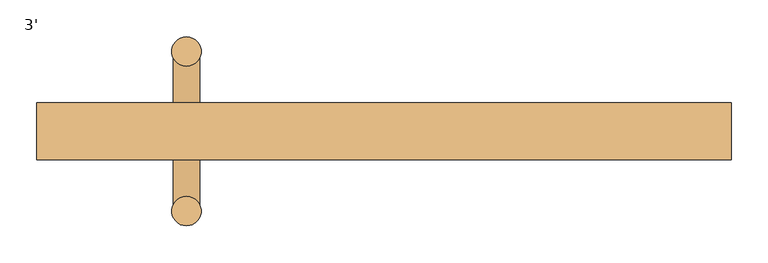
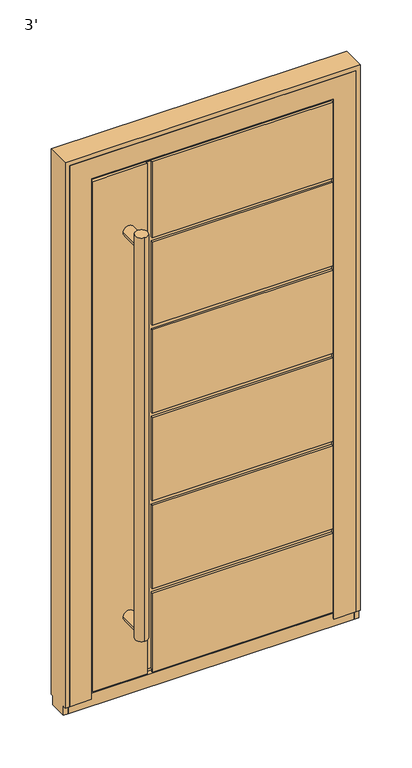
"""IFC4 building model written with IfcOpenShell, lengths in millimetres: door geometry, 3'."""

from ifc_helpers import new_model, si_unit, point, frame, frame_2d, origin, place, context, project, spatial, circle_curve, trimmed, segment, composite_curve, outline, extrude, faceted_brep, source, transform, mapped, element, save


def door_3_ad1505b7(model_context):
    return source(origin(), model_context, "Body", "SolidModel", [
        extrude(outline(composite_curve([segment(trimmed(circle_curve(frame_2d((-268.65, -90.8003001)), 20.0), [point((-268.65, -70.8003001))], [point((-268.65, -110.8003001))], False, "CARTESIAN"), True, "CONTINUOUS"), segment(trimmed(circle_curve(frame_2d((-268.65, -90.8003001)), 20.0), [point((-268.65, -110.8003001))], [point((-268.65, -70.8003001))], False, "CARTESIAN"), True, "CONTINUOUS")], self_intersect=False)), frame((0.0, 0.0, 210.0000003), z_axis=(0.0, 0.0, 1.0), x_axis=(1.0, 0.0, 0.0)), (0.0, 0.0, 1.0), 1363.8),
        extrude(outline(composite_curve([segment(trimmed(circle_curve(frame_2d((-268.65, 126.2003001)), 20.0), [point((-268.65, 146.2003001))], [point((-268.65, 106.2003001))], False, "CARTESIAN"), True, "CONTINUOUS"), segment(trimmed(circle_curve(frame_2d((-268.65, 126.2003001)), 20.0), [point((-268.65, 106.2003001))], [point((-268.65, 146.2003001))], False, "CARTESIAN"), True, "CONTINUOUS")], self_intersect=False)), frame((0.0, 0.0, 210.0000003), z_axis=(0.0, 0.0, 1.0), x_axis=(1.0, 0.0, 0.0)), (0.0, 0.0, 1.0), 1363.8),
        extrude(outline(composite_curve([segment(trimmed(circle_curve(frame_2d((241.9000003, -268.65)), 18.0), [point((241.9000003, -286.65))], [point((241.9000003, -250.65))], False, "CARTESIAN"), True, "CONTINUOUS"), segment(trimmed(circle_curve(frame_2d((241.9000003, -268.65)), 18.0), [point((241.9000003, -250.65))], [point((241.9000003, -286.65))], False, "CARTESIAN"), True, "CONTINUOUS")], self_intersect=False)), frame((0.0, -90.8, 0.0), z_axis=(0.0, 1.0, 0.0), x_axis=(0.0, 0.0, 1.0)), (0.0, 0.0, 1.0), 217.0),
        extrude(outline(composite_curve([segment(trimmed(circle_curve(frame_2d((1541.9000003, -268.65)), 18.0), [point((1541.9000003, -286.65))], [point((1541.9000003, -250.65))], False, "CARTESIAN"), True, "CONTINUOUS"), segment(trimmed(circle_curve(frame_2d((1541.9000003, -268.65)), 18.0), [point((1541.9000003, -250.65))], [point((1541.9000003, -286.65))], False, "CARTESIAN"), True, "CONTINUOUS")], self_intersect=False)), frame((0.0, -90.8, 0.0), z_axis=(0.0, 1.0, 0.0), x_axis=(0.0, 0.0, 1.0)), (0.0, 0.0, 1.0), 217.0),
        faceted_brep([(-193.65, -13.8, 306.466667), (-193.65, -13.8, 587.9333337), (383.65, -13.8, 587.9333337), (383.65, -13.8, 602.9333337), (-193.65, -13.8, 602.9333337), (-193.65, -13.8, 884.4000004), (383.65, -13.8, 884.4000004), (383.65, -13.8, 899.4000004), (-193.65, -13.8, 899.4000004), (-193.65, -13.8, 1180.866667), (383.65, -13.8, 1180.866667), (383.65, -13.8, 1195.866667), (-193.65, -13.8, 1195.866667), (-193.65, -13.8, 1477.3333337), (383.65, -13.8, 1477.3333337), (383.65, -13.8, 1492.3333337), (-193.65, -13.8, 1492.3333337), (-193.65, -13.8, 1748.8000003), (-208.65, -13.8, 1748.8000003), (-208.65, -13.8, 35.0), (-193.65, -13.8, 35.0), (-193.65, -13.8, 291.466667), (383.65, -13.8, 291.466667), (383.65, -13.8, 306.466667), (-193.65, -20.8, 306.466667), (-193.65, -20.8, 587.9333337), (383.65, -20.8, 587.9333337), (383.65, -11.7997698, 1748.8000003), (383.65, -20.8, 1748.8000003), (383.65, -20.8, 1492.3333337), (383.65, -20.8, 1477.3333337), (383.65, -20.8, 1195.866667), (383.65, -20.8, 1180.866667), (383.65, -20.8, 899.4000004), (383.65, -20.8, 884.4000004), (383.65, -20.8, 602.9333337), (383.65, -20.8, 306.466667), (383.65, -20.8, 291.466667), (383.65, -20.8, 24.0), (383.65, -18.8020472, 24.0), (383.65, -18.8020472, 35.0), (383.65, -11.7997698, 35.0), (-193.65, -20.8, 602.9333337), (-193.65, -20.8, 884.4000004), (-193.65, -20.8, 899.4000004), (-193.65, -20.8, 1180.866667), (-208.65, -20.8, 1748.8000003), (-208.65, -20.8, 24.0), (-208.65, -18.8020472, 24.0), (-208.65, -18.8020472, 35.0), (-193.65, -18.8020472, 35.0), (-383.65, -18.8020472, 35.0), (-383.65, -11.7997698, 35.0), (-193.65, -20.8, 291.466667), (-193.65, -18.8020472, 24.0), (-193.65, -20.8, 24.0), (-383.65, -18.8020472, 24.0), (-383.65, -20.8, 24.0), (-383.65, -20.8, 1748.8000003), (-193.65, -20.8, 1477.3333337), (-193.65, -20.8, 1195.866667), (-193.65, -20.8, 1748.8000003), (-193.65, -20.8, 1492.3333337), (408.65, 56.2, 10.0000003), (408.65, 53.2, 10.0000003), (-193.65, 53.2, 10.0000003), (-193.65, 56.2, 10.0000003), (-408.65, 53.2, 10.0000003), (-408.65, 56.2, 10.0000003), (-208.65, 56.2, 10.0000003), (-208.65, 53.2, 10.0000003), (408.65, 56.2, 291.466667), (408.65, 53.2, 291.466667), (408.65, 56.2, 306.466667), (408.65, 56.2, 587.9333337), (408.65, 53.2, 587.9333337), (408.65, 53.2, 306.466667), (408.65, 56.2, 899.4000004), (408.65, 56.2, 1180.866667), (408.65, 53.2, 1180.866667), (408.65, 53.2, 899.4000004), (408.65, 56.2, 602.9333337), (408.65, 56.2, 884.4000004), (408.65, 53.2, 884.4000004), (408.65, 53.2, 602.9333337), (408.65, 56.2, 1195.866667), (408.65, 56.2, 1477.3333337), (408.65, 53.2, 1477.3333337), (408.65, 53.2, 1195.866667), (408.65, 56.2, 1773.8000003), (408.65, 53.2, 1773.8000003), (408.65, 53.2, 1492.3333337), (408.65, 56.2, 1492.3333337), (393.15, 53.2, 291.466667), (393.15, 53.2, 25.5), (-193.65, 53.2, 25.5), (393.15, 53.2, 587.9333337), (393.15, 53.2, 306.466667), (393.15, 53.2, 1180.866667), (393.15, 53.2, 899.4000004), (393.15, 53.2, 884.4000004), (393.15, 53.2, 602.9333337), (393.15, 53.2, 1477.3333337), (393.15, 53.2, 1195.866667), (-193.65, 53.2, 1773.8000003), (-193.65, 53.2, 1758.3000003), (393.15, 53.2, 1758.3000003), (393.15, 53.2, 1492.3333337), (-393.15, 53.2, 25.5), (-393.15, 53.2, 1758.3000003), (-208.65, 53.2, 1758.3000003), (-208.65, 53.2, 1773.8000003), (-408.65, 53.2, 1773.8000003), (-208.65, 53.2, 25.5), (-193.65, 49.2, 291.466667), (-193.65, 56.2, 291.466667), (-193.65, 49.2, 25.5), (-193.65, 56.2, 306.466667), (-193.65, 56.2, 587.9333337), (-193.65, 56.2, 899.4000004), (-193.65, 56.2, 1180.866667), (-193.65, 56.2, 602.9333337), (-193.65, 56.2, 884.4000004), (-193.65, 56.2, 1195.866667), (-193.65, 56.2, 1477.3333337), (-193.65, 56.2, 1492.3333337), (-193.65, 56.2, 1773.8000003), (-408.65, 56.2, 1773.8000003), (-208.65, 56.2, 1773.8000003), (-208.65, 49.2, 1758.3000003), (-208.65, 49.2, 25.5), (-383.65, -11.7997698, 1748.8000003), (393.15, -11.7997698, 1758.3000003), (-393.15, -11.7997698, 1758.3000003), (-393.15, -11.7997698, 25.5), (393.15, -11.7997698, 25.5), (393.15, 49.2, 291.466667), (393.15, 49.2, 306.466667), (393.15, 49.2, 587.9333337), (393.15, 49.2, 602.9333337), (393.15, 49.2, 884.4000004), (393.15, 49.2, 899.4000004), (393.15, 49.2, 1180.866667), (393.15, 49.2, 1195.866667), (393.15, 49.2, 1477.3333337), (393.15, 49.2, 1492.3333337), (-193.65, 49.2, 1477.3333337), (-193.65, 49.2, 1195.866667), (-193.65, 49.2, 1180.866667), (-193.65, 49.2, 899.4000004), (-193.65, 49.2, 884.4000004), (-193.65, 49.2, 602.9333337), (-193.65, 49.2, 587.9333337), (-193.65, 49.2, 306.466667), (-193.65, 49.2, 1758.3000003), (-193.65, 49.2, 1492.3333337)], [[[0, 1, 2, 3, 4, 5, 6, 7, 8, 9, 10, 11, 12, 13, 14, 15, 16, 17, 18, 19, 20, 21, 22, 23]], [[1, 0, 24, 25]], [[1, 25, 26, 2]], [[27, 28, 29, 15, 14, 30, 31, 11, 10, 32, 33, 7, 6, 34, 35, 3, 2, 26, 36, 23, 22, 37, 38, 39, 40, 41]], [[42, 4, 3, 35]], [[5, 4, 42, 43]], [[5, 43, 34, 6]], [[44, 8, 7, 33]], [[9, 8, 44, 45]], [[19, 18, 46, 47, 48, 49]], [[41, 40, 50, 20, 19, 49, 51, 52]], [[53, 21, 20, 50, 54, 55]], [[21, 53, 37, 22]], [[24, 0, 23, 36]], [[40, 39, 54, 50]], [[56, 51, 49, 48]], [[39, 38, 55, 54]], [[57, 56, 48, 47]], [[33, 32, 45, 44]], [[35, 34, 43, 42]], [[36, 26, 25, 24]], [[55, 38, 37, 53]], [[58, 57, 47, 46]], [[31, 30, 59, 60]], [[28, 61, 62, 29]], [[63, 64, 65, 66]], [[67, 68, 69, 70]], [[64, 63, 71, 72]], [[73, 74, 75, 76]], [[77, 78, 79, 80]], [[81, 82, 83, 84]], [[85, 86, 87, 88]], [[89, 90, 91, 92]], [[65, 64, 72, 93, 94, 95]], [[76, 75, 96, 97]], [[80, 79, 98, 99]], [[84, 83, 100, 101]], [[88, 87, 102, 103]], [[90, 104, 105, 106, 107, 91]], [[108, 109, 110, 111, 112, 67, 70, 113]], [[114, 115, 66, 65, 95, 116]], [[63, 66, 115, 71]], [[74, 73, 117, 118]], [[78, 77, 119, 120]], [[82, 81, 121, 122]], [[86, 85, 123, 124]], [[89, 92, 125, 126]], [[68, 127, 128, 69]], [[68, 67, 112, 127]], [[129, 130, 113, 70, 69, 128, 111, 110]], [[58, 131, 52, 51, 56, 57]], [[132, 133, 134, 135], [131, 27, 41, 52]], [[106, 132, 135, 94, 93, 136, 137, 97, 96, 138, 139, 101, 100, 140, 141, 99, 98, 142, 143, 103, 102, 144, 145, 107]], [[94, 135, 134, 108, 113, 130, 116, 95]], [[133, 109, 108, 134]], [[146, 147, 143, 142, 148, 149, 141, 140, 150, 151, 139, 138, 152, 153, 137, 136, 114, 116, 130, 129, 154, 155, 145, 144]], [[149, 148, 120, 119]], [[149, 119, 77, 80, 99, 141]], [[122, 150, 140, 100, 83, 82]], [[151, 150, 122, 121]], [[151, 121, 81, 84, 101, 139]], [[118, 152, 138, 96, 75, 74]], [[153, 152, 118, 117]], [[153, 117, 73, 76, 97, 137]], [[115, 114, 136, 93, 72, 71]], [[9, 45, 32, 10]], [[60, 12, 11, 31]], [[13, 12, 60, 59]], [[13, 59, 30, 14]], [[62, 16, 15, 29]], [[16, 62, 61, 17]], [[124, 146, 144, 102, 87, 86]], [[125, 155, 154, 105, 104, 126]], [[120, 148, 142, 98, 79, 78]], [[147, 123, 85, 88, 103, 143]], [[147, 146, 124, 123]], [[155, 125, 92, 91, 107, 145]], [[90, 89, 126, 104]], [[127, 112, 111, 128]], [[132, 106, 105, 154, 129, 110, 109, 133]], [[27, 131, 58, 46, 18, 17, 61, 28]]]),
        faceted_brep([(-457.2, 56.2, 0.0), (-412.7, 56.2, 0.0), (-412.7, 47.2, 0.0), (-457.2, 47.1997571, 0.0), (-403.2, -16.2999958, 0.0), (-387.7, -16.2999958, 0.0), (-387.7, -20.8, 0.0), (-457.2, -20.8, 0.0), (-457.2, -11.8, 0.0), (-403.2, -11.8, 0.0), (457.2, -20.8, 0.0), (387.7, -20.8, 0.0), (387.7, -16.2999958, 0.0), (403.2, -16.2999958, 0.0), (403.2, -11.8, 0.0), (457.2, -11.8, 0.0), (412.7, 47.2, 0.0), (412.7, 56.2, 0.0), (457.2, 56.2, 0.0), (457.2, 47.1997571, 0.0), (-457.2, -20.8, 1828.8), (-457.2, 56.2, 1828.8), (-457.2, 47.1997571, -30.0), (-457.2, -11.8, -30.0), (457.2, 56.2, 1828.8), (412.7, 56.2, 1784.3), (-412.7, 56.2, 1784.3), (457.2, -20.8, 1828.8), (457.2, -11.8, -30.0), (457.2, 47.1997571, -30.0), (-387.7, -20.8, 1759.3), (387.7, -20.8, 1759.3), (-403.2, 47.2, 1774.8), (-403.2, -16.2999958, 1774.8), (-403.2, -11.8, 14.5), (-403.2, 47.2, 14.5), (403.2, 47.2, 1774.8), (403.2, -16.2999958, 1774.8), (403.2, 47.2, 14.5), (403.2, -11.8, 14.5), (-412.7, 47.2, 1784.3), (412.7, 47.2, 1784.3), (387.7, -16.2999958, 1759.3), (-387.7, -16.2999958, 1759.3)], [[[0, 1, 2, 3]], [[4, 5, 6, 7, 8, 9]], [[10, 11, 12, 13, 14, 15]], [[16, 17, 18, 19]], [[7, 20, 21, 0, 3, 22, 23, 8]], [[1, 0, 21, 24, 18, 17, 25, 26]], [[21, 20, 27, 24]], [[18, 24, 27, 10, 15, 28, 29, 19]], [[7, 6, 30, 31, 11, 10, 27, 20]], [[32, 33, 4, 9, 34, 35]], [[33, 32, 36, 37]], [[37, 36, 38, 39, 14, 13]], [[40, 2, 1, 26]], [[16, 19, 29, 22, 3, 2, 40, 41], [36, 32, 35, 38]], [[5, 4, 33, 37, 13, 12, 42, 43]], [[6, 5, 43, 30]], [[26, 25, 41, 40]], [[31, 30, 43, 42]], [[17, 16, 41, 25]], [[12, 11, 31, 42]], [[23, 28, 15, 14, 39, 34, 9, 8]], [[38, 35, 34, 39]], [[23, 22, 29, 28]]]),
        faceted_brep([(-457.2, 47.2, -30.0), (-457.2, -11.8, -30.0), (-472.2, -11.8, -30.0), (-472.2, 47.2, -30.0), (-457.2, 56.2, 1828.8), (-457.2, -20.8, 1828.8), (-457.2, -20.8, 0.0), (-457.2, -11.8, 0.0), (-457.2, 47.2, 0.0), (-457.2, 56.2, 0.0), (472.2, -11.8, 0.0), (457.2, -11.8, 0.0), (457.2, -11.8, -30.0), (472.2, -11.8, -30.0), (-472.2, -11.8, 0.0), (-472.2, -20.8, 1843.8), (-472.2, 56.2, 1843.8), (-472.2, 56.2, 0.0), (-472.2, 47.2, 0.0), (-472.2, -20.8, 0.0), (457.2, 47.2, 0.0), (472.2, 47.2, 0.0), (472.2, 47.2, -30.0), (457.2, 47.2, -30.0), (457.2, -20.8, 1828.8), (457.2, 56.2, 1828.8), (457.2, 56.2, 0.0), (457.2, -20.8, 0.0), (472.2, 56.2, 1843.8), (472.2, 56.2, 0.0), (472.2, -20.8, 0.0), (472.2, -20.8, 1843.8)], [[[0, 1, 2, 3]], [[4, 5, 6, 7, 1, 0, 8, 9]], [[10, 11, 12, 13]], [[7, 14, 2, 1]], [[15, 16, 17, 18, 3, 2, 14, 19]], [[20, 21, 22, 23]], [[18, 8, 0, 3]], [[24, 25, 26, 20, 23, 12, 11, 27]], [[25, 4, 9, 17, 16, 28, 29, 26]], [[21, 20, 26, 29]], [[8, 18, 17, 9]], [[22, 13, 12, 23]], [[11, 10, 30, 27]], [[14, 7, 6, 19]], [[5, 24, 27, 30, 31, 15, 19, 6]], [[28, 31, 30, 10, 13, 22, 21, 29]], [[5, 4, 25, 24]], [[16, 15, 31, 28]]]),
    ])


if __name__ == "__main__":
    model = new_model("IFC4")
    model_context = context("Model", 3, world=origin())
    ifc_project = project(units=[si_unit("LENGTHUNIT", "METRE", prefix="MILLI")], contexts=[model_context])
    site = spatial("IfcSite", under=ifc_project)
    building = spatial("IfcBuilding", under=site)
    placement = place(None, origin())
    door_3_shape = door_3_ad1505b7(model_context)
    element("IfcDoor", 1, ObjectType="3'", at=placement, inside=building, context=model_context, shape_type="MappedRepresentation", body=[
        mapped(door_3_shape, transform((0.0, 0.0, 0.0), x_axis=(1.0, 0.0, 0.0), y_axis=(0.0, 1.0, 0.0), z_axis=(0.0, 0.0, 1.0))),
    ])
    save(model, "model.ifc")

# Revit data of these elements
# Type "3'"
#   Type Mark = "9"
#   Water resistance = "up to Class E900, EN 12208:2001"
#   Uniclass2015Version = "v1.21"
#   Uniclass2015Reference = "Ss_25_30_20_30"
#   Uniclass2015Description = "Frame and door leaf system"
#   URL = "www.aluprof.com"
#   Type IFC Predefined Type = "USERDEFINED"
#   Right-hand / Left-hand door [instance default] = ""
#   Resistance to wind load = "up to Class C5/B5, EN 12210:2001"
#   Insert type = "ST"
#   Hardware [instance default] = ""
#   Product page = "https://aluprof.com/en/architects/offer/window-and-door-systems/panel-doors#visualisation"
#   Operation = "SinglePanelOutwardOpening"
#   Opening type = "Outward"
#   NBSReference = "25-50-20/125"
#   NBSDescription = "Frame and door leaf system"
#   Important = "The actual acceptable construction dimensions are dependent on the selection of profiles and hardware, glazing type, construction weight and the construction’s operating conditions. These should be determined by a suitably qualified person, and using ALUPROF’s calculation software"
#   IfcExportType = "USERDEFINED"
#   IfcExportAs = "IfcDoorType"
#   Handle type [instance default] = ""
#   Manufacturer = "ALUPROF SA"
#   Export Type to IFC As = "IfcDoorType"
#   Door sill type [instance default] = ""
#   Description = "External single-leaf panel door outward opening"
#   Model = "MB-86 ST Panel Door AD07"
#   Content of the recyclate in the material = "69.2%"
#   COBie.Type.WarrantyDurationParts = ""
#   COBie.Type.Name = ""
#   COBie.Type.Manufacturer = "ALUPROF SA"
#   COBie.Space.Name = ""
#   COBie.Floor.Name = ""
#   COBie.Facility.Name = ""
#   COBie.CreatedOn = ""
#   COBie.Component.WarrantyStartDate = ""
#   COBie.Component.Name = "MB-86 ST Panel Door AD07"
#   Burglar resistance = "RC2"
#   Air permeability = "up to Class 4, EN 12207:2001"
#   Width of the active leaf = 2' - 8.17717"
#   Placement in wall = 0' - 0.7874"
#   Thickness = 0' - 3.0315"
#   Height of the opening sash = 5' - 9.44094"
#   Handle Offset = 3' - 5.33858"
#   Rough Height = 6' - 2.40945"
#   Rough Width = 3' - 1.1811"
#   Height = 6' - 0"
#   Width = 3' - 0"
#   Construction depth = 0' - 3.0315"
#   Clear opening width = 2' - 3.94882"
#   Clear opening height = 5' - 8.47638"
#   Height of the array = 0' - 11.08136"
#   Schedule No. [instance default] = 1
#   Handrail [instance default] = yes
#   IsExternal = yes
#   Handle [instance default] = no
#   Door closer [instance default] = no
#   Function = 1
#   COBie.Type = yes
#   COBie = yes
#   Access control [instance default] = no
#   Panel = element 380783
#   Wall Closure = (empty or 0)
